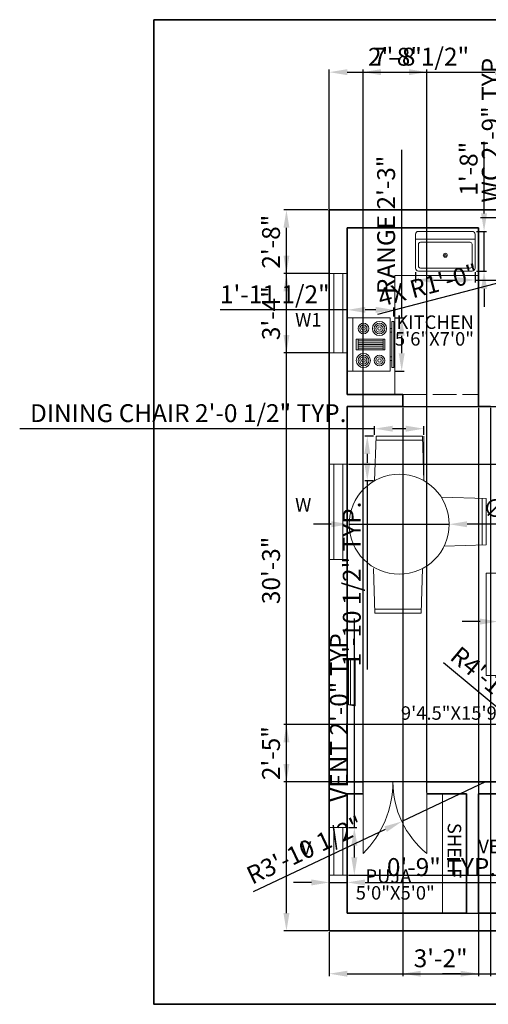
# Model space of a CAD drawing. Units: inches. Extents: x 1838 to 3181, y 1882 to 2430.
# Tile 1 of 4: x 1838 to 2073, y 1894 to 2389. Entities that reach past the tile are written whole.
import ezdxf

# ---------------------------------------------------------------- set-up
doc = ezdxf.new("R2010")
doc.units = ezdxf.units.IN
doc.linetypes.add('ACAD_ISO02W100', pattern=[15, 12, -3])
for name, color, linetype, lineweight in [('A-ANNO-TEXT', 7, 'Continuous', 18), ('A-ANNO-TTLB', 7, 'Continuous', 35), ('A-AREA-IDEN', 7, 'Continuous', 18), ('A-DOOR', 4, 'Continuous', 18), ('A-EQPM', 9, 'Continuous', 18), ('A-FLOR-CASE', 8, 'Continuous', 18), ('A-FLOR-FIXT', 9, 'Continuous', 18), ('A-FURN', 8, 'Continuous', 18), ('A-GLAZ', 11, 'Continuous', 18), ('A-WALL', 7, 'Continuous', 35), ('A-WALL-OVHD', 7, 'ACAD_ISO02W100', 18), ('S-ANNO-DIMS', 2, 'Continuous', 18)]:
    doc.layers.add(name, color=color, linetype=linetype, lineweight=lineweight)
doc.styles.get("Standard").update_dxf_attribs({"font": 'arial.ttf'})
doc.dimstyles.new('ISO-25', dxfattribs={"dimtxt": 9, "dimasz": 9, "dimexe": 1.25, "dimexo": 0.625, "dimgap": 2, "dimtad": 1, "dimdec": 1, "dimlunit": 4, "dimtxsty": 'Standard', "dimcen": 2.5, "dimadec": 0, "dimazin": 0, "dimtfac": 1, "dimtdec": 1, "dimtmove": 0, "dimatfit": 3, "dimfxl": 1, "dimarcsym": 0})

# ---------------------------------------------------------------- blocks, each defined once
blk = doc.blocks.new('Range-Oven - 30 in top')
for p, q in [((0, -3), (30, -3)), ((12, -6), (18, -6)), ((13, -20), (13, -6)), ((14, -6), (14, -20)), ((15, -20), (15, -6)), ((16, -6), (16, -20)), ((17, -20), (17, -6)), ((18, -20), (12, -20)), ((6, -24), (6, -25)), ((8, -25), (8, -24)), ((22, -25), (22, -24)), ((24, -24), (24, -25))]:
    blk.add_line(p, q)
for points in [[(0, -24), (0, 0), (30, 0), (30, -24)], [(12, -21), (12, -5), (18, -5), (18, -21)], [(2, -26), (2, -25), (28, -25), (28, -26)]]:
    blk.add_lwpolyline(points, close=True)
for centre, radius in [((6, -9), 4), ((6, -9), 3), ((6, -9), 2), ((6, -9), 1), ((24, -9), 3), ((24, -9), 2), ((24, -9), 1), ((6, -18), 3), ((6, -18), 2), ((24, -18), 4), ((24, -18), 3), ((24, -18), 2), ((6, -18), 1), ((24, -18), 1)]:
    blk.add_circle(centre, radius)
blk = doc.blocks.new('Sink-single - 30 in top')
blk.add_line((-15, -3.999996), (15, -3.999996))
for points in [[(-13.5, 0), (13.5, 0)], [(-15, -18.499996), (-15, -1.5)], [(15, -1.5), (15, -18.499996)], [(-13.5, -17.499996), (-13.5, -6.499996)], [(-12.5, -5.499996), (12.5, -5.499996)], [(13.5, -6.499996), (13.5, -17.499996)], [(12.5, -18.499996), (-12.5, -18.499996)], [(13.5, -19.999996), (-13.5, -19.999996)]]:
    blk.add_lwpolyline(points)
for radius in [1, 0.5]:
    blk.add_circle((0, -11.999996), radius)
for centre, radius, start, end in [((-13.5, -1.5), 1.5, 90, 180), ((13.5, -1.5), 1.5, 0, 90), ((-12.5, -6.499996), 1, 90, 180), ((12.5, -6.499996), 1, 0, 90), ((-13.5, -18.499996), 1.5, 180, 270), ((-12.5, -17.499996), 1, 180, 270), ((12.5, -17.499996), 1, 270, 0), ((13.5, -18.499996), 1.5, 270, 0)]:
    blk.add_arc(centre, radius, start, end)
blk = doc.blocks.new('WIN-48')
for p, q in [((0, 48), (9, 48)), ((2.25, 48), (2.25, 0)), ((6.75, 48), (6.75, 0)), ((0, 0), (9, 0))]:
    blk.add_line(p, q)
blk = doc.blocks.new('VENT-24')
for p, q in [((0, 24), (9, 24)), ((2.25, 24), (2.25, 0)), ((6.75, 24), (6.75, 0)), ((0, 0), (9, 0))]:
    blk.add_line(p, q)
blk = doc.blocks.new('CHAIR-DINING')
for p, q in [((0, 22.48), (0.69, 0)), ((24.67, 22.48), (23.99, 0)), ((23.99, 2), (0.69, 2)), ((23.99, 0), (0.69, 0))]:
    blk.add_line(p, q)
blk = doc.blocks.new('*D25')
at = {"layer": 'Defpoints', "color": 0, "transparency": 16777216}
for p in [(2002.53, 1982.46), (2006.13, 1982.46), (2002.53, 1958.46)]:
    blk.add_point(p, dxfattribs=at)
at = {"layer": 'S-ANNO-DIMS', "color": 0, "lineweight": -2, "transparency": 16777216}
for p, q in [((2006.13, 1982.46), (2006.13, 2087.81)), ((2003.16, 1982.46), (2007.38, 1982.46)), ((2006.13, 1967.46), (2006.13, 1973.46)), ((2003.16, 1958.46), (2007.38, 1958.46))]:
    blk.add_line(p, q, dxfattribs=at)
at = {"layer": 'S-ANNO-DIMS', "color": 0, "transparency": 16777216}
for points in [[(2004.63, 1973.46), (2007.63, 1973.46), (2006.13, 1982.46)], [(2004.63, 1967.46), (2007.63, 1967.46), (2006.13, 1958.46)]]:
    blk.add_solid(points, dxfattribs=at)
at = {"layer": 'S-ANNO-DIMS', "color": 0, "transparency": 16777216, "insert": (1999.54, 2039.63), "char_height": 9, "attachment_point": 5, "rotation": 90}
blk.add_mtext('VENT 2\'-0" TYP.', dxfattribs=at)
blk = doc.blocks.new('*D26')
at = {"layer": 'Defpoints', "color": 0, "transparency": 16777216}
for p in [(1993.53, 1958.46), (2002.53, 1958.46), (2002.53, 1954.86)]:
    blk.add_point(p, dxfattribs=at)
at = {"layer": 'S-ANNO-DIMS', "color": 0, "lineweight": -2, "transparency": 16777216}
for p, q in [((1984.53, 1954.86), (1975.53, 1954.86)), ((1993.53, 1957.83), (1993.53, 1953.61)), ((1993.53, 1954.86), (2002.53, 1954.86)), ((2002.53, 1957.83), (2002.53, 1953.61)), ((2011.53, 1954.86), (2079.39, 1954.86))]:
    blk.add_line(p, q, dxfattribs=at)
at = {"layer": 'S-ANNO-DIMS', "color": 0, "transparency": 16777216}
for points in [[(1984.53, 1956.36), (1984.53, 1953.36), (1993.53, 1954.86)], [(2011.53, 1956.36), (2011.53, 1953.36), (2002.53, 1954.86)]]:
    blk.add_solid(points, dxfattribs=at)
at = {"layer": 'S-ANNO-DIMS', "color": 0, "transparency": 16777216, "insert": (2049.96, 1961.45), "char_height": 9, "attachment_point": 5}
blk.add_mtext('0\'-9" TYP.', dxfattribs=at)
blk = doc.blocks.new('*D31')
at = {"layer": 'Defpoints', "color": 0, "transparency": 16777216}
for p in [(2082.53, 2284.46), (2087.49, 2284.46), (2087.49, 2251.41)]:
    blk.add_point(p, dxfattribs=at)
at = {"layer": 'S-ANNO-DIMS', "color": 0, "lineweight": -2, "transparency": 16777216}
for p, q in [((2082.53, 2284.46), (2082.53, 2377.12)), ((2086.87, 2284.46), (2081.28, 2284.46)), ((2082.53, 2260.41), (2082.53, 2275.46)), ((2086.87, 2251.41), (2081.28, 2251.41))]:
    blk.add_line(p, q, dxfattribs=at)
at = {"layer": 'S-ANNO-DIMS', "color": 0, "transparency": 16777216}
for points in [[(2081.03, 2275.46), (2084.03, 2275.46), (2082.53, 2284.46)], [(2081.03, 2260.41), (2084.03, 2260.41), (2082.53, 2251.41)]]:
    blk.add_solid(points, dxfattribs=at)
at = {"layer": 'S-ANNO-DIMS', "color": 0, "transparency": 16777216, "insert": (2075.88, 2335.29), "char_height": 9, "attachment_point": 5, "rotation": 90}
blk.add_mtext('WC 2\'-9" TYP.', dxfattribs=at)
blk = doc.blocks.new('*D32')
at = {"layer": 'Defpoints', "color": 0, "transparency": 16777216}
for p in [(2108.49, 2289.41), (2087.49, 2284.46), (2108.49, 2284.46)]:
    blk.add_point(p, dxfattribs=at)
at = {"layer": 'S-ANNO-DIMS', "color": 0, "lineweight": -2, "transparency": 16777216}
for p, q in [((2087.49, 2285.08), (2087.49, 2290.66)), ((2108.49, 2285.08), (2108.49, 2290.66)), ((2078.49, 2289.41), (2069.49, 2289.41)), ((2087.49, 2289.41), (2108.49, 2289.41)), ((2117.49, 2289.41), (2184.5, 2289.41))]:
    blk.add_line(p, q, dxfattribs=at)
at = {"layer": 'S-ANNO-DIMS', "color": 0, "transparency": 16777216}
for points in [[(2078.49, 2290.91), (2078.49, 2287.91), (2087.49, 2289.41)], [(2117.49, 2290.91), (2117.49, 2287.91), (2108.49, 2289.41)]]:
    blk.add_solid(points, dxfattribs=at)
at = {"layer": 'S-ANNO-DIMS', "color": 0, "transparency": 16777216, "insert": (2155.5, 2296.01), "char_height": 9, "attachment_point": 5}
blk.add_mtext('1\'-9" TYP.', dxfattribs=at)
blk = doc.blocks.new('*D33')
at = {"layer": 'Defpoints', "color": 0, "transparency": 16777216}
for p in [(2016.34, 2183.31), (2016.34, 2179.61), (2041.01, 2179.61)]:
    blk.add_point(p, dxfattribs=at)
at = {"layer": 'S-ANNO-DIMS', "color": 0, "lineweight": -2, "transparency": 16777216}
for p, q in [((2016.34, 2183.31), (1837.85, 2183.31)), ((2016.34, 2180.24), (2016.34, 2184.56)), ((2032.01, 2183.31), (2025.34, 2183.31)), ((2041.01, 2180.24), (2041.01, 2184.56))]:
    blk.add_line(p, q, dxfattribs=at)
at = {"layer": 'S-ANNO-DIMS', "color": 0, "transparency": 16777216}
for points in [[(2025.34, 2184.81), (2025.34, 2181.81), (2016.34, 2183.31)], [(2032.01, 2184.81), (2032.01, 2181.81), (2041.01, 2183.31)]]:
    blk.add_solid(points, dxfattribs=at)
at = {"layer": 'S-ANNO-DIMS', "color": 0, "transparency": 16777216, "insert": (1922.6, 2189.97), "char_height": 9, "attachment_point": 5}
blk.add_mtext('DINING CHAIR 2\'-0 1/2" TYP.', dxfattribs=at)
blk = doc.blocks.new('*D34')
at = {"layer": 'Defpoints', "color": 0, "transparency": 16777216}
for p in [(2016.34, 2179.61), (2012.64, 2157.13), (2016.34, 2157.13)]:
    blk.add_point(p, dxfattribs=at)
at = {"layer": 'S-ANNO-DIMS', "color": 0, "lineweight": -2, "transparency": 16777216}
for p, q in [((2015.72, 2179.61), (2011.39, 2179.61)), ((2012.64, 2170.61), (2012.64, 2166.13)), ((2015.72, 2157.13), (2011.39, 2157.13)), ((2012.64, 2157.13), (2012.64, 2062.15))]:
    blk.add_line(p, q, dxfattribs=at)
at = {"layer": 'S-ANNO-DIMS', "color": 0, "transparency": 16777216}
for points in [[(2011.14, 2170.61), (2014.14, 2170.61), (2012.64, 2179.61)], [(2011.14, 2166.13), (2014.14, 2166.13), (2012.64, 2157.13)]]:
    blk.add_solid(points, dxfattribs=at)
at = {"layer": 'S-ANNO-DIMS', "color": 0, "transparency": 16777216, "insert": (2005.99, 2105.14), "char_height": 9, "attachment_point": 5, "rotation": 90}
blk.add_mtext('1\'-10 1/2" TYP.', dxfattribs=at)
blk = doc.blocks.new('*D35')
at = {"layer": 'Defpoints', "color": 0, "transparency": 16777216}
for p in [(2025.9, 2239.11), (2029.93, 2239.11), (2025.9, 2212.28)]:
    blk.add_point(p, dxfattribs=at)
at = {"layer": 'S-ANNO-DIMS', "color": 0, "lineweight": -2, "transparency": 16777216}
for p, q in [((2029.93, 2239.11), (2029.93, 2323.77)), ((2026.53, 2239.11), (2031.18, 2239.11)), ((2029.93, 2221.28), (2029.93, 2230.11)), ((2026.53, 2212.28), (2031.18, 2212.28))]:
    blk.add_line(p, q, dxfattribs=at)
at = {"layer": 'S-ANNO-DIMS', "color": 0, "transparency": 16777216}
for points in [[(2028.43, 2230.11), (2031.43, 2230.11), (2029.93, 2239.11)], [(2028.43, 2221.28), (2031.43, 2221.28), (2029.93, 2212.28)]]:
    blk.add_solid(points, dxfattribs=at)
at = {"layer": 'S-ANNO-DIMS', "color": 0, "transparency": 16777216, "insert": (2023.27, 2285.94), "char_height": 9, "attachment_point": 5, "rotation": 90}
blk.add_mtext('RANGE 2\'-3"', dxfattribs=at)
blk = doc.blocks.new('*D36')
at = {"layer": 'Defpoints', "color": 0, "transparency": 16777216}
for p in [(2002.65, 2243.13), (2002.65, 2239.11), (2025.9, 2239.11)]:
    blk.add_point(p, dxfattribs=at)
at = {"layer": 'S-ANNO-DIMS', "color": 0, "lineweight": -2, "transparency": 16777216}
for p, q in [((2002.65, 2243.13), (1938.61, 2243.13)), ((2002.65, 2239.73), (2002.65, 2244.38)), ((2016.9, 2243.13), (2011.65, 2243.13)), ((2025.9, 2239.73), (2025.9, 2244.38))]:
    blk.add_line(p, q, dxfattribs=at)
at = {"layer": 'S-ANNO-DIMS', "color": 0, "transparency": 16777216}
for points in [[(2011.65, 2244.63), (2011.65, 2241.63), (2002.65, 2243.13)], [(2016.9, 2244.63), (2016.9, 2241.63), (2025.9, 2243.13)]]:
    blk.add_solid(points, dxfattribs=at)
at = {"layer": 'S-ANNO-DIMS', "color": 0, "transparency": 16777216, "insert": (1966.13, 2249.79), "char_height": 9, "attachment_point": 5}
blk.add_mtext('1\'-11 1/2"', dxfattribs=at)
blk = doc.blocks.new('*D37')
at = {"layer": 'Defpoints', "color": 0, "transparency": 16777216}
for p in [(2036.86, 2262.67), (2066.86, 2262.67), (2066.86, 2258.17)]:
    blk.add_point(p, dxfattribs=at)
at = {"layer": 'S-ANNO-DIMS', "color": 0, "lineweight": -2, "transparency": 16777216}
for p, q in [((2036.86, 2262.04), (2036.86, 2256.92)), ((2066.86, 2262.04), (2066.86, 2256.92)), ((2045.86, 2258.17), (2057.86, 2258.17)), ((2066.86, 2258.17), (2136.58, 2258.17))]:
    blk.add_line(p, q, dxfattribs=at)
at = {"layer": 'S-ANNO-DIMS', "color": 0, "transparency": 16777216}
for points in [[(2045.86, 2259.67), (2045.86, 2256.67), (2036.86, 2258.17)], [(2057.86, 2259.67), (2057.86, 2256.67), (2066.86, 2258.17)]]:
    blk.add_solid(points, dxfattribs=at)
at = {"layer": 'S-ANNO-DIMS', "color": 0, "transparency": 16777216, "insert": (2106.22, 2264.82), "char_height": 9, "attachment_point": 5}
blk.add_mtext('SINK 2\'-6"', dxfattribs=at)
blk = doc.blocks.new('*D38')
at = {"layer": 'Defpoints', "color": 0, "transparency": 16777216}
for p in [(2066.86, 2282.67), (2071.36, 2282.67), (2066.86, 2262.67)]:
    blk.add_point(p, dxfattribs=at)
at = {"layer": 'S-ANNO-DIMS', "color": 0, "lineweight": -2, "transparency": 16777216}
for p, q in [((2071.36, 2291.67), (2071.36, 2327.74)), ((2067.48, 2282.67), (2072.61, 2282.67)), ((2071.36, 2262.67), (2071.36, 2282.67)), ((2067.48, 2262.67), (2072.61, 2262.67)), ((2071.36, 2253.67), (2071.36, 2244.67))]:
    blk.add_line(p, q, dxfattribs=at)
at = {"layer": 'S-ANNO-DIMS', "color": 0, "transparency": 16777216}
for points in [[(2069.86, 2291.67), (2072.86, 2291.67), (2071.36, 2282.67)], [(2069.86, 2253.67), (2072.86, 2253.67), (2071.36, 2262.67)]]:
    blk.add_solid(points, dxfattribs=at)
at = {"layer": 'S-ANNO-DIMS', "color": 0, "transparency": 16777216, "insert": (2064.76, 2314.2), "char_height": 9, "attachment_point": 5, "rotation": 90}
blk.add_mtext('1\'-8"', dxfattribs=at)
blk = doc.blocks.new('*D39')
at = {"layer": 'Defpoints', "color": 0, "transparency": 16777216}
for p in [(1993.53, 1930.46), (2243.53, 1930.46), (2243.53, 1908.91)]:
    blk.add_point(p, dxfattribs=at)
at = {"layer": 'S-ANNO-DIMS', "color": 0, "lineweight": -2, "transparency": 16777216}
for p, q in [((1993.53, 1929.83), (1993.53, 1907.66)), ((2243.53, 1929.83), (2243.53, 1907.66)), ((2002.53, 1908.91), (2234.53, 1908.91))]:
    blk.add_line(p, q, dxfattribs=at)
at = {"layer": 'S-ANNO-DIMS', "color": 0, "transparency": 16777216}
for points in [[(2002.53, 1910.41), (2002.53, 1907.41), (1993.53, 1908.91)], [(2234.53, 1910.41), (2234.53, 1907.41), (2243.53, 1908.91)]]:
    blk.add_solid(points, dxfattribs=at)
at = {"layer": 'S-ANNO-DIMS', "color": 0, "transparency": 16777216, "insert": (2118.53, 1915.5), "char_height": 9, "attachment_point": 5}
blk.add_mtext('20\'-10"', dxfattribs=at)
blk = doc.blocks.new('*D40')
at = {"layer": 'Defpoints', "color": 0, "transparency": 16777216}
for p in [(1971.98, 2293.46), (1993.53, 2293.46), (1993.53, 1930.46)]:
    blk.add_point(p, dxfattribs=at)
at = {"layer": 'S-ANNO-DIMS', "color": 0, "lineweight": -2, "transparency": 16777216}
for p, q in [((1992.91, 2293.46), (1970.73, 2293.46)), ((1971.98, 1939.46), (1971.98, 2284.46)), ((1992.91, 1930.46), (1970.73, 1930.46))]:
    blk.add_line(p, q, dxfattribs=at)
at = {"layer": 'S-ANNO-DIMS', "color": 0, "transparency": 16777216}
for points in [[(1970.48, 2284.46), (1973.48, 2284.46), (1971.98, 2293.46)], [(1970.48, 1939.46), (1973.48, 1939.46), (1971.98, 1930.46)]]:
    blk.add_solid(points, dxfattribs=at)
at = {"layer": 'S-ANNO-DIMS', "color": 0, "transparency": 16777216, "insert": (1965.39, 2111.96), "char_height": 9, "attachment_point": 5, "rotation": 90}
blk.add_mtext('30\'-3"', dxfattribs=at)
blk = doc.blocks.new('*D41')
at = {"layer": 'Defpoints', "color": 0, "transparency": 16777216}
for p in [(2002.53, 1958.46), (2265.08, 1958.46), (2002.53, 1939.46)]:
    blk.add_point(p, dxfattribs=at)
at = {"layer": 'S-ANNO-DIMS', "color": 0, "lineweight": -2, "transparency": 16777216}
for p, q in [((2265.08, 1967.46), (2265.08, 2003.53)), ((2003.16, 1958.46), (2266.33, 1958.46)), ((2265.08, 1939.46), (2265.08, 1958.46)), ((2003.16, 1939.46), (2266.33, 1939.46)), ((2265.08, 1930.46), (2265.08, 1921.46))]:
    blk.add_line(p, q, dxfattribs=at)
at = {"layer": 'S-ANNO-DIMS', "color": 0, "transparency": 16777216}
for points in [[(2263.58, 1967.46), (2266.58, 1967.46), (2265.08, 1958.46)], [(2263.58, 1930.46), (2266.58, 1930.46), (2265.08, 1939.46)]]:
    blk.add_solid(points, dxfattribs=at)
at = {"layer": 'S-ANNO-DIMS', "color": 0, "transparency": 16777216, "insert": (2258.57, 1989.99), "char_height": 9, "attachment_point": 5, "rotation": 90}
blk.add_mtext('1\'-7"', dxfattribs=at)
blk = doc.blocks.new('*D42')
at = {"layer": 'Defpoints', "color": 0, "transparency": 16777216}
for p in [(2002.53, 2194.46), (2265.08, 2194.46), (2002.53, 2165.46)]:
    blk.add_point(p, dxfattribs=at)
at = {"layer": 'S-ANNO-DIMS', "color": 0, "lineweight": -2, "transparency": 16777216}
for p, q in [((2003.16, 2194.46), (2266.33, 2194.46)), ((2265.08, 2174.46), (2265.08, 2185.46)), ((2003.16, 2165.46), (2266.33, 2165.46))]:
    blk.add_line(p, q, dxfattribs=at)
at = {"layer": 'S-ANNO-DIMS', "color": 0, "transparency": 16777216}
for points in [[(2263.58, 2185.46), (2266.58, 2185.46), (2265.08, 2194.46)], [(2263.58, 2174.46), (2266.58, 2174.46), (2265.08, 2165.46)]]:
    blk.add_solid(points, dxfattribs=at)
at = {"layer": 'S-ANNO-DIMS', "color": 0, "transparency": 16777216, "insert": (2258.49, 2179.96), "char_height": 9, "attachment_point": 5, "rotation": 90}
blk.add_mtext('2\'-5"', dxfattribs=at)
blk = doc.blocks.new('*D43')
at = {"layer": 'Defpoints', "color": 0, "transparency": 16777216}
for p in [(1971.98, 2293.46), (1993.53, 2293.46), (1993.53, 2261.46)]:
    blk.add_point(p, dxfattribs=at)
at = {"layer": 'S-ANNO-DIMS', "color": 0, "lineweight": -2, "transparency": 16777216}
for p, q in [((1992.91, 2293.46), (1970.73, 2293.46)), ((1971.98, 2270.46), (1971.98, 2284.46)), ((1992.91, 2261.46), (1970.73, 2261.46))]:
    blk.add_line(p, q, dxfattribs=at)
at = {"layer": 'S-ANNO-DIMS', "color": 0, "transparency": 16777216}
for points in [[(1970.48, 2284.46), (1973.48, 2284.46), (1971.98, 2293.46)], [(1970.48, 2270.46), (1973.48, 2270.46), (1971.98, 2261.46)]]:
    blk.add_solid(points, dxfattribs=at)
at = {"layer": 'S-ANNO-DIMS', "color": 0, "transparency": 16777216, "insert": (1965.39, 2277.46), "char_height": 9, "attachment_point": 5, "rotation": 90}
blk.add_mtext('2\'-8"', dxfattribs=at)
blk = doc.blocks.new('*D44')
at = {"layer": 'Defpoints', "color": 0, "transparency": 16777216}
for p in [(1971.98, 2261.46), (1993.53, 2261.46), (1993.53, 2221.46)]:
    blk.add_point(p, dxfattribs=at)
at = {"layer": 'S-ANNO-DIMS', "color": 0, "lineweight": -2, "transparency": 16777216}
for p, q in [((1992.91, 2261.46), (1970.73, 2261.46)), ((1971.98, 2230.46), (1971.98, 2252.46)), ((1992.91, 2221.46), (1970.73, 2221.46))]:
    blk.add_line(p, q, dxfattribs=at)
at = {"layer": 'S-ANNO-DIMS', "color": 0, "transparency": 16777216}
for points in [[(1970.48, 2252.46), (1973.48, 2252.46), (1971.98, 2261.46)], [(1970.48, 2230.46), (1973.48, 2230.46), (1971.98, 2221.46)]]:
    blk.add_solid(points, dxfattribs=at)
at = {"layer": 'S-ANNO-DIMS', "color": 0, "transparency": 16777216, "insert": (1965.39, 2241.46), "char_height": 9, "attachment_point": 5, "rotation": 90}
blk.add_mtext('3\'-4"', dxfattribs=at)
blk = doc.blocks.new('*D45')
at = {"layer": 'Defpoints', "color": 0, "transparency": 16777216}
for p in [(1971.98, 2034.46), (2234.53, 2034.46), (2234.53, 2005.46)]:
    blk.add_point(p, dxfattribs=at)
at = {"layer": 'S-ANNO-DIMS', "color": 0, "lineweight": -2, "transparency": 16777216}
for p, q in [((2233.91, 2034.46), (1970.73, 2034.46)), ((1971.98, 2014.46), (1971.98, 2025.46)), ((2233.91, 2005.46), (1970.73, 2005.46))]:
    blk.add_line(p, q, dxfattribs=at)
at = {"layer": 'S-ANNO-DIMS', "color": 0, "transparency": 16777216}
for points in [[(1970.48, 2025.46), (1973.48, 2025.46), (1971.98, 2034.46)], [(1970.48, 2014.46), (1973.48, 2014.46), (1971.98, 2005.46)]]:
    blk.add_solid(points, dxfattribs=at)
at = {"layer": 'S-ANNO-DIMS', "color": 0, "transparency": 16777216, "insert": (1965.39, 2019.96), "char_height": 9, "attachment_point": 5, "rotation": 90}
blk.add_mtext('2\'-5"', dxfattribs=at)
blk = doc.blocks.new('*D48')
at = {"layer": 'Defpoints', "color": 0, "transparency": 16777216}
for p in [(2085.84, 2362.82), (1993.53, 2293.46), (2085.84, 2293.46)]:
    blk.add_point(p, dxfattribs=at)
at = {"layer": 'S-ANNO-DIMS', "color": 0, "lineweight": -2, "transparency": 16777216}
for p, q in [((1993.53, 2294.08), (1993.53, 2364.07)), ((2002.53, 2362.82), (2076.84, 2362.82)), ((2085.84, 2294.08), (2085.84, 2364.07))]:
    blk.add_line(p, q, dxfattribs=at)
at = {"layer": 'S-ANNO-DIMS', "color": 0, "transparency": 16777216}
for points in [[(2002.53, 2364.32), (2002.53, 2361.32), (1993.53, 2362.82)], [(2076.84, 2364.32), (2076.84, 2361.32), (2085.84, 2362.82)]]:
    blk.add_solid(points, dxfattribs=at)
at = {"layer": 'S-ANNO-DIMS', "color": 0, "transparency": 16777216, "insert": (2039.69, 2369.47), "char_height": 9, "attachment_point": 5}
blk.add_mtext('7\'-8 1/2"', dxfattribs=at)
blk = doc.blocks.new('*D52')
at = {"layer": 'Defpoints', "color": 0, "transparency": 16777216}
for p in [(2042.53, 2362.82), (2010.53, 1999.46), (2042.53, 1999.46)]:
    blk.add_point(p, dxfattribs=at)
at = {"layer": 'S-ANNO-DIMS', "color": 0, "lineweight": -2, "transparency": 16777216}
for p, q in [((2010.53, 2000.08), (2010.53, 2364.07)), ((2019.53, 2362.82), (2033.53, 2362.82)), ((2042.53, 2000.08), (2042.53, 2364.07))]:
    blk.add_line(p, q, dxfattribs=at)
at = {"layer": 'S-ANNO-DIMS', "color": 0, "transparency": 16777216}
for points in [[(2019.53, 2364.32), (2019.53, 2361.32), (2010.53, 2362.82)], [(2033.53, 2364.32), (2033.53, 2361.32), (2042.53, 2362.82)]]:
    blk.add_solid(points, dxfattribs=at)
at = {"layer": 'S-ANNO-DIMS', "color": 0, "transparency": 16777216, "insert": (2026.53, 2369.41), "char_height": 9, "attachment_point": 5}
blk.add_mtext('2\'-8"', dxfattribs=at)
blk = doc.blocks.new('*D54')
at = {"layer": 'Defpoints', "color": 0, "transparency": 16777216}
for p in [(2030.53, 2194.46), (2068.53, 2194.46), (2068.53, 1908.91)]:
    blk.add_point(p, dxfattribs=at)
at = {"layer": 'S-ANNO-DIMS', "color": 0, "lineweight": -2, "transparency": 16777216}
for p, q in [((2030.53, 2193.83), (2030.53, 1907.66)), ((2068.53, 2193.83), (2068.53, 1907.66)), ((2039.53, 1908.91), (2059.53, 1908.91))]:
    blk.add_line(p, q, dxfattribs=at)
at = {"layer": 'S-ANNO-DIMS', "color": 0, "transparency": 16777216}
for points in [[(2039.53, 1910.41), (2039.53, 1907.41), (2030.53, 1908.91)], [(2059.53, 1910.41), (2059.53, 1907.41), (2068.53, 1908.91)]]:
    blk.add_solid(points, dxfattribs=at)
at = {"layer": 'S-ANNO-DIMS', "color": 0, "transparency": 16777216, "insert": (2049.53, 1915.5), "char_height": 9, "attachment_point": 5}
blk.add_mtext('3\'-2"', dxfattribs=at)
blk = doc.blocks.new('*D55')
at = {"layer": 'Defpoints', "color": 0, "transparency": 16777216}
for p in [(2068.53, 2194.46), (2074.53, 2194.46), (2074.53, 1908.91)]:
    blk.add_point(p, dxfattribs=at)
at = {"layer": 'S-ANNO-DIMS', "color": 0, "lineweight": -2, "transparency": 16777216}
for p, q in [((2068.53, 2193.83), (2068.53, 1907.66)), ((2074.53, 2193.83), (2074.53, 1907.66)), ((2059.53, 1908.91), (2050.53, 1908.91)), ((2068.53, 1908.91), (2074.53, 1908.91)), ((2083.53, 1908.91), (2120.46, 1908.91))]:
    blk.add_line(p, q, dxfattribs=at)
at = {"layer": 'S-ANNO-DIMS', "color": 0, "transparency": 16777216}
for points in [[(2059.53, 1910.41), (2059.53, 1907.41), (2068.53, 1908.91)], [(2083.53, 1910.41), (2083.53, 1907.41), (2074.53, 1908.91)]]:
    blk.add_solid(points, dxfattribs=at)
at = {"layer": 'S-ANNO-DIMS', "color": 0, "transparency": 16777216, "insert": (2106.5, 1915.5), "char_height": 9, "attachment_point": 5}
blk.add_mtext('0\'-6"', dxfattribs=at)
blk = doc.blocks.new('*D68')
at = {"layer": 'Defpoints', "color": 0, "transparency": 16777216}
for p in [(2003.51, 2135.2), (2053.84, 2135.2)]:
    blk.add_point(p, dxfattribs=at)
at = {"layer": 'S-ANNO-DIMS', "color": 0, "lineweight": -2, "transparency": 16777216}
for p, q in [((1994.51, 2135.2), (1985.51, 2135.2)), ((2003.51, 2135.2), (2053.84, 2135.2)), ((2130.53, 2135.2), (2062.84, 2135.2))]:
    blk.add_line(p, q, dxfattribs=at)
at = {"layer": 'S-ANNO-DIMS', "color": 0, "transparency": 16777216}
for points in [[(1994.51, 2136.7), (1994.51, 2133.7), (2003.51, 2135.2)], [(2062.84, 2136.7), (2062.84, 2133.7), (2053.84, 2135.2)]]:
    blk.add_solid(points, dxfattribs=at)
at = {"layer": 'S-ANNO-DIMS', "color": 0, "transparency": 16777216, "insert": (2101.19, 2142.04), "char_height": 9, "attachment_point": 5, "rotation": 359.9991}
blk.add_mtext('∅4\'-2 1/2"', dxfattribs=at)
blk = doc.blocks.new('*D69')
at = {"layer": 'Defpoints', "color": 0, "transparency": 16777216}
for p in [(2078.35, 2086.21), (2088.77, 2086.21)]:
    blk.add_point(p, dxfattribs=at)
at = {"layer": 'S-ANNO-DIMS', "color": 0, "lineweight": -2, "transparency": 16777216}
for p, q in [((2069.35, 2086.21), (2060.35, 2086.21)), ((2078.35, 2086.21), (2088.77, 2086.21)), ((2172.45, 2086.22), (2097.77, 2086.21))]:
    blk.add_line(p, q, dxfattribs=at)
at = {"layer": 'S-ANNO-DIMS', "color": 0, "transparency": 16777216}
for points in [[(2069.35, 2087.71), (2069.35, 2084.71), (2078.35, 2086.21)], [(2097.77, 2087.71), (2097.77, 2084.71), (2088.77, 2086.21)]]:
    blk.add_solid(points, dxfattribs=at)
at = {"layer": 'S-ANNO-DIMS', "color": 0, "transparency": 16777216, "insert": (2139.61, 2093.06), "char_height": 9, "attachment_point": 5, "rotation": 0.0024}
blk.add_mtext('∅0\'-10 1/2"', dxfattribs=at)
blk = doc.blocks.new('*D70')
at = {"layer": 'Defpoints', "color": 0, "transparency": 16777216}
for p in [(2092.84, 2030.7), (2130.33, 1999.46)]:
    blk.add_point(p, dxfattribs=at)
at = {"layer": 'S-ANNO-DIMS', "color": 0, "lineweight": -2, "transparency": 16777216}
for p, q in [((2050.95, 2065.61), (2085.93, 2036.46)), ((2130.33, 1999.46), (2092.84, 2030.7))]:
    blk.add_line(p, q, dxfattribs=at)
at = {"layer": 'S-ANNO-DIMS', "color": 0, "transparency": 16777216}
blk.add_solid([(2086.89, 2037.61), (2084.97, 2035.31), (2092.84, 2030.7)], dxfattribs=at)
at = {"layer": 'S-ANNO-DIMS', "color": 0, "transparency": 16777216, "insert": (2069.16, 2058.92), "char_height": 9, "attachment_point": 5, "rotation": 320.1941}
blk.add_mtext('R4\'-1"', dxfattribs=at)
blk = doc.blocks.new('*D71')
at = {"layer": 'Defpoints', "color": 0, "transparency": 16777216}
for p in [(2072.15, 2005.46), (2030, 1985.55)]:
    blk.add_point(p, dxfattribs=at)
at = {"layer": 'S-ANNO-DIMS', "color": 0, "lineweight": -2, "transparency": 16777216}
for p, q in [((2072.15, 2005.46), (2030, 1985.55)), ((1955.4, 1950.32), (2021.86, 1981.71))]:
    blk.add_line(p, q, dxfattribs=at)
at = {"layer": 'S-ANNO-DIMS', "color": 0, "transparency": 16777216}
blk.add_solid([(2021.22, 1983.06), (2022.5, 1980.35), (2030, 1985.55)], dxfattribs=at)
at = {"layer": 'S-ANNO-DIMS', "color": 0, "transparency": 16777216, "insert": (1981.72, 1970.11), "char_height": 9, "attachment_point": 5, "rotation": 25.2778}
blk.add_mtext('R3\'-10 1/2"', dxfattribs=at)
blk = doc.blocks.new('*D74')
at = {"layer": 'Defpoints', "color": 0, "transparency": 16777216}
for p in [(2101.51, 2262.88), (2089.74, 2259.78)]:
    blk.add_point(p, dxfattribs=at)
at = {"layer": 'S-ANNO-DIMS', "color": 0, "lineweight": -2, "transparency": 16777216}
for p, q in [((2101.51, 2262.88), (2089.74, 2259.78)), ((2017.94, 2240.92), (2081.04, 2257.5))]:
    blk.add_line(p, q, dxfattribs=at)
at = {"layer": 'S-ANNO-DIMS', "color": 0, "transparency": 16777216}
blk.add_solid([(2080.65, 2258.95), (2081.42, 2256.05), (2089.74, 2259.78)], dxfattribs=at)
at = {"layer": 'S-ANNO-DIMS', "color": 0, "transparency": 16777216, "insert": (2043.46, 2254.44), "char_height": 9, "attachment_point": 5, "rotation": 14.7211}
blk.add_mtext('4X R1\'-0"', dxfattribs=at)

msp = doc.modelspace()

# ---------------------------------------------------------------- linework, layer by layer
at = {"layer": 'A-ANNO-TTLB'}
msp.add_lwpolyline([(1905.37, 2389.23), (3180.85, 2389.23), (3180.85, 1893.51), (1905.37, 1893.51)], close=True, dxfattribs=at)
at = {"layer": 'A-DOOR'}
for p, q in [((2010.53, 2005.46), (2010.53, 1969.46)), ((2042.53, 2005.46), (2042.53, 1969.46))]:
    msp.add_line(p, q, dxfattribs=at)
for centre, radius, start, end in [((1974.83, 2005.46), 50.7, 314.7603, 0), ((2072.15, 2005.46), 46.62, 180, 230.5554)]:
    msp.add_arc(centre, radius, start, end, dxfattribs=at)
at = {"layer": 'A-EQPM'}
for p, q in [((2003.23, 2067.25), (2006.23, 2067.75)), ((2003.23, 2067.25), (2003.23, 2044.25)), ((2003.23, 2067.25), (2006.23, 2067.25)), ((2004.23, 2067.25), (2004.23, 2044.25)), ((2006.23, 2067.75), (2006.53, 2067.75)), ((2006.23, 2067.25), (2006.23, 2044.25)), ((2006.53, 2067.75), (2006.53, 2043.75)), ((2003.23, 2044.25), (2006.23, 2044.25)), ((2003.23, 2044.25), (2006.23, 2043.75)), ((2006.23, 2043.75), (2006.53, 2043.75))]:
    msp.add_line(p, q, dxfattribs=at)
at = {"layer": 'A-FLOR-CASE'}
for p, q in [((2026.53, 2260.46), (2068.53, 2260.46)), ((2026.53, 2260.46), (2026.53, 2200.46)), ((2050.53, 1999.46), (2050.53, 1939.46))]:
    msp.add_line(p, q, dxfattribs=at)
at = {"layer": 'A-FURN'}
for p, q in [((2041.01, 2157.13), (2041.01, 2179.61)), ((2049.82, 2148.88), (2072.45, 2148.19)), ((2070.45, 2148.19), (2070.45, 2124.9)), ((2072.45, 2148.19), (2072.45, 2124.9)), ((2051.33, 2124.25), (2072.45, 2124.9))]:
    msp.add_line(p, q, dxfattribs=at)
msp.add_lwpolyline([(2072.38, 2110.61), (2094.15, 2110.61), (2094.15, 2059.05), (2072.38, 2059.05)], close=True, dxfattribs=at)
msp.add_circle((2028.68, 2135.2), 25.16, dxfattribs=at)
at = {"layer": 'A-GLAZ'}
for p, q in [((1993.53, 2261.46), (2002.53, 2261.46)), ((1995.78, 2261.46), (1995.78, 2221.46)), ((2000.28, 2261.46), (2000.28, 2221.46)), ((1993.53, 2221.46), (2002.53, 2221.46)), ((1995.78, 1982.46), (1995.78, 1958.46)), ((2000.28, 1982.46), (2000.28, 1958.46))]:
    msp.add_line(p, q, dxfattribs=at)
at = {"layer": 'A-WALL'}
for p, q in [((1993.53, 2293.46), (2243.53, 2293.46)), ((1993.53, 2293.46), (1993.53, 1930.46)), ((2002.53, 2284.46), (2068.53, 2284.46)), ((2002.53, 2284.46), (2002.53, 2200.46)), ((2002.53, 2284.46), (2002.53, 2200.46)), ((2068.53, 2284.46), (2068.53, 2194.46)), ((2002.53, 2200.46), (2030.53, 2200.46)), ((2030.53, 2200.46), (2030.53, 2194.46)), ((2002.53, 2194.46), (2030.53, 2194.46)), ((2002.53, 2194.46), (2002.53, 2005.46)), ((2068.53, 2194.46), (2074.53, 2194.46)), ((2002.53, 2005.46), (2010.53, 2005.46)), ((2042.53, 2005.46), (2081.53, 2005.46)), ((2002.53, 1999.46), (2010.53, 1999.46)), ((2002.53, 1999.46), (2002.53, 1939.46)), ((2042.53, 1999.46), (2062.53, 1999.46)), ((2062.53, 1999.46), (2062.53, 1939.46)), ((2068.53, 1999.46), (2068.53, 1939.46)), ((2068.53, 1999.46), (2081.53, 1999.46)), ((2002.53, 1939.46), (2062.53, 1939.46)), ((2068.53, 1939.46), (2234.53, 1939.46)), ((1993.53, 1930.46), (2243.53, 1930.46))]:
    msp.add_line(p, q, dxfattribs=at)
at = {"layer": 'A-WALL-OVHD'}
for p, q in [((2030.53, 2200.46), (2068.53, 2200.46)), ((2030.53, 2194.46), (2074.53, 2194.46))]:
    msp.add_line(p, q, dxfattribs=at)

# ---------------------------------------------------------------- block references
at = {"layer": 'A-EQPM', "xscale": 0.8944271909999159, "yscale": 0.8944271909999159, "zscale": 0.8944271909999159, "rotation": 89.99999999999999}
msp.add_blockref('Range-Oven - 30 in top', (2002.65, 2212.28), dxfattribs=at)
at = {"layer": 'A-FLOR-FIXT'}
msp.add_blockref('Sink-single - 30 in top', (2051.86, 2282.67), dxfattribs=at)
at = {"layer": 'A-FURN', "rotation": 180}
msp.add_blockref('CHAIR-DINING', (2041.01, 2179.61), dxfattribs=at)
at = {"layer": 'A-FURN'}
msp.add_blockref('CHAIR-DINING', (2015.75, 2090.46), dxfattribs=at)
at = {"layer": 'A-GLAZ', "rotation": 180}
msp.add_blockref('WIN-48', (2002.53, 2165.46), dxfattribs=at)
at = {"layer": 'A-GLAZ'}
msp.add_blockref('VENT-24', (1993.53, 1958.46), dxfattribs=at)

# ---------------------------------------------------------------- texts
at = {"layer": 'A-ANNO-TEXT'}
for s, height, p in [('W1', 6.784, (1976.36, 2234.74)), ('W', 6.78, (1976.36, 2141.6)), ('V', 6.78, (1979.16, 1968.77))]:
    msp.add_text(s, height=height, dxfattribs=at).set_placement(p)
msp.add_text('SHELF', height=6.784, rotation=270, dxfattribs=at).set_placement((2053.07, 1984.85))
at = {"layer": 'A-AREA-IDEN'}
for s, height, p in [('KITCHEN', 6.784, (2027.24, 2233.55)), (' 5\'6"X7\'0"', 6.784, (2024.44, 2225.14)), ('    9\'4.5"X15\'9"', 6.7841, (2021.24, 2036.76)), ('VERANDAH', 6.784, (2068.46, 1969.58)), ('  PUJA', 6.784, (2007.55, 1954.64)), (' 5\'0"X5\'0"', 6.784, (2004.74, 1946.24))]:
    msp.add_text(s, height=height, dxfattribs=at).set_placement(p)

# ---------------------------------------------------------------- dimensions: what is measured, and where the dimension line sits
at = {"layer": 'S-ANNO-DIMS'}
for base, p1, p2, picture, middle in [((2085.84, 2362.82), (1993.53, 2293.46), (2085.84, 2293.46), '*D48', (2039.69, 2369.47)), ((2042.53, 2362.82), (2010.53, 1999.46), (2042.53, 1999.46), '*D52', (2026.53, 2369.41)), ((2068.53, 1908.91), (2030.53, 2194.46), (2068.53, 2194.46), '*D54', (2049.53, 1915.5)), ((2074.53, 1908.91), (2068.53, 2194.46), (2074.53, 2194.46), '*D55', (2106.5, 1915.5)), ((2243.53, 1908.91), (1993.53, 1930.46), (2243.53, 1930.46), '*D39', (2118.53, 1915.5))]:
    dim = msp.add_linear_dim(base=base, p1=p1, p2=p2, dimstyle='ISO-25', override={"dimdec": 1, "dimlfac": 1, "dimrnd": 0, "dimzin": 1, "dimdsep": 46, "dimlunit": 4, "dimfrac": 2}, dxfattribs=at)
    dim.commit()
    dim.dimension.update_dxf_attribs({"geometry": picture, "text_midpoint": middle})
for base, p1, p2, angle, text, picture, middle in [((2082.5334, 2284.4559), (2087.4904, 2251.4097), (2087.4904, 2284.4559), 90, 'WC <> TYP.', '*D31', (2075.8799, 2335.2898)), ((2029.93, 2239.11), (2025.9, 2212.28), (2025.9, 2239.11), 90, 'RANGE <>', '*D35', (2023.27, 2285.94)), ((2016.34, 2183.31), (2041.01, 2179.61), (2016.34, 2179.61), 180, 'DINING CHAIR <> TYP.', '*D33', (1922.6, 2189.97)), ((2012.64, 2157.13), (2016.34, 2179.61), (2016.34, 2157.13), 270, '<> TYP.', '*D34', (2005.99, 2105.14)), ((2006.13, 1982.46), (2002.53, 1958.46), (2002.53, 1982.46), 90, 'VENT <> TYP.', '*D25', (1999.54, 2039.63))]:
    dim = msp.add_linear_dim(base=base, p1=p1, p2=p2, angle=angle, text=text, dimstyle='ISO-25', override={"dimdec": 1, "dimlfac": 1, "dimrnd": 0, "dimzin": 1, "dimdsep": 46, "dimlunit": 4, "dimfrac": 2}, dxfattribs=at)
    dim.commit()
    dim.dimension.update_dxf_attribs({"geometry": picture, "text_midpoint": middle})
for base, p1, p2, angle, picture, middle in [((2071.36, 2282.67), (2066.86, 2262.67), (2066.86, 2282.67), 90, '*D38', (2064.76, 2314.2)), ((1971.98, 2293.46), (1993.53, 1930.46), (1993.53, 2293.46), 90, '*D40', (1965.39, 2111.96)), ((1971.98, 2293.46), (1993.53, 2261.46), (1993.53, 2293.46), 90, '*D43', (1965.39, 2277.46)), ((2002.6474, 2243.1341), (2025.9025, 2239.1091), (2002.6474, 2239.1091), 180, '*D36', (1966.127, 2249.7875)), ((1971.98, 2261.46), (1993.53, 2221.46), (1993.53, 2261.46), 90, '*D44', (1965.39, 2241.46)), ((2265.08, 2194.46), (2002.53, 2165.46), (2002.53, 2194.46), 90, '*D42', (2258.49, 2179.96)), ((1971.98, 2034.46), (2234.53, 2005.46), (2234.53, 2034.46), 90, '*D45', (1965.39, 2019.96)), ((2265.08, 1958.46), (2002.53, 1939.46), (2002.53, 1958.46), 90, '*D41', (2258.57, 1989.99))]:
    dim = msp.add_linear_dim(base=base, p1=p1, p2=p2, angle=angle, dimstyle='ISO-25', override={"dimdec": 1, "dimlfac": 1, "dimrnd": 0, "dimzin": 1, "dimdsep": 46, "dimlunit": 4, "dimfrac": 2}, dxfattribs=at)
    dim.commit()
    dim.dimension.update_dxf_attribs({"geometry": picture, "text_midpoint": middle})
for base, p1, p2, text, picture, middle in [((2108.49, 2289.41), (2087.49, 2284.46), (2108.49, 2284.46), '<> TYP.', '*D32', (2155.5, 2296.01)), ((2066.86, 2258.17), (2036.86, 2262.67), (2066.86, 2262.67), 'SINK <>', '*D37', (2106.22, 2264.82)), ((2002.53, 1954.86), (1993.53, 1958.46), (2002.53, 1958.46), '<> TYP.', '*D26', (2049.96, 1961.45))]:
    dim = msp.add_linear_dim(base=base, p1=p1, p2=p2, text=text, dimstyle='ISO-25', override={"dimdec": 1, "dimlfac": 1, "dimrnd": 0, "dimzin": 1, "dimdsep": 46, "dimlunit": 4, "dimfrac": 2}, dxfattribs=at)
    dim.commit()
    dim.dimension.update_dxf_attribs({"geometry": picture, "text_midpoint": middle})
dim = msp.add_radius_dim(center=(2101.51, 2262.88), mpoint=(2089.74, 2259.78), text='4X <>', dimstyle='ISO-25', override={"dimdec": 1, "dimlfac": 1, "dimrnd": 0, "dimzin": 1, "dimdsep": 46, "dimlunit": 4, "dimfrac": 2}, dxfattribs=at)
dim.commit()
dim.dimension.update_dxf_attribs({"geometry": '*D74', "text_midpoint": (2043.46, 2254.44)})
for p1, p2, picture, middle in [((2003.51, 2135.2), (2053.84, 2135.2), '*D68', (2101.19, 2135.2)), ((2078.35, 2086.21), (2088.77, 2086.21), '*D69', (2139.61, 2086.22))]:
    dim = msp.add_diameter_dim_2p(p1=p1, p2=p2, dimstyle='ISO-25', override={"dimdec": 1, "dimlfac": 1, "dimrnd": 0, "dimzin": 1, "dimdsep": 46, "dimlunit": 4, "dimfrac": 2}, dxfattribs=at)
    dim.commit()
    dim.dimension.update_dxf_attribs({"geometry": picture, "text_midpoint": middle})
for center, mpoint, picture, middle in [((2130.33, 1999.46), (2092.84, 2030.7), '*D70', (2069.16, 2058.92)), ((2072.15, 2005.46), (2030, 1985.55), '*D71', (1981.72, 1970.11))]:
    dim = msp.add_radius_dim(center=center, mpoint=mpoint, dimstyle='ISO-25', override={"dimdec": 1, "dimlfac": 1, "dimrnd": 0, "dimzin": 1, "dimdsep": 46, "dimlunit": 4, "dimfrac": 2}, dxfattribs=at)
    dim.commit()
    dim.dimension.update_dxf_attribs({"geometry": picture, "text_midpoint": middle})

doc.saveas('drawing.dxf')
